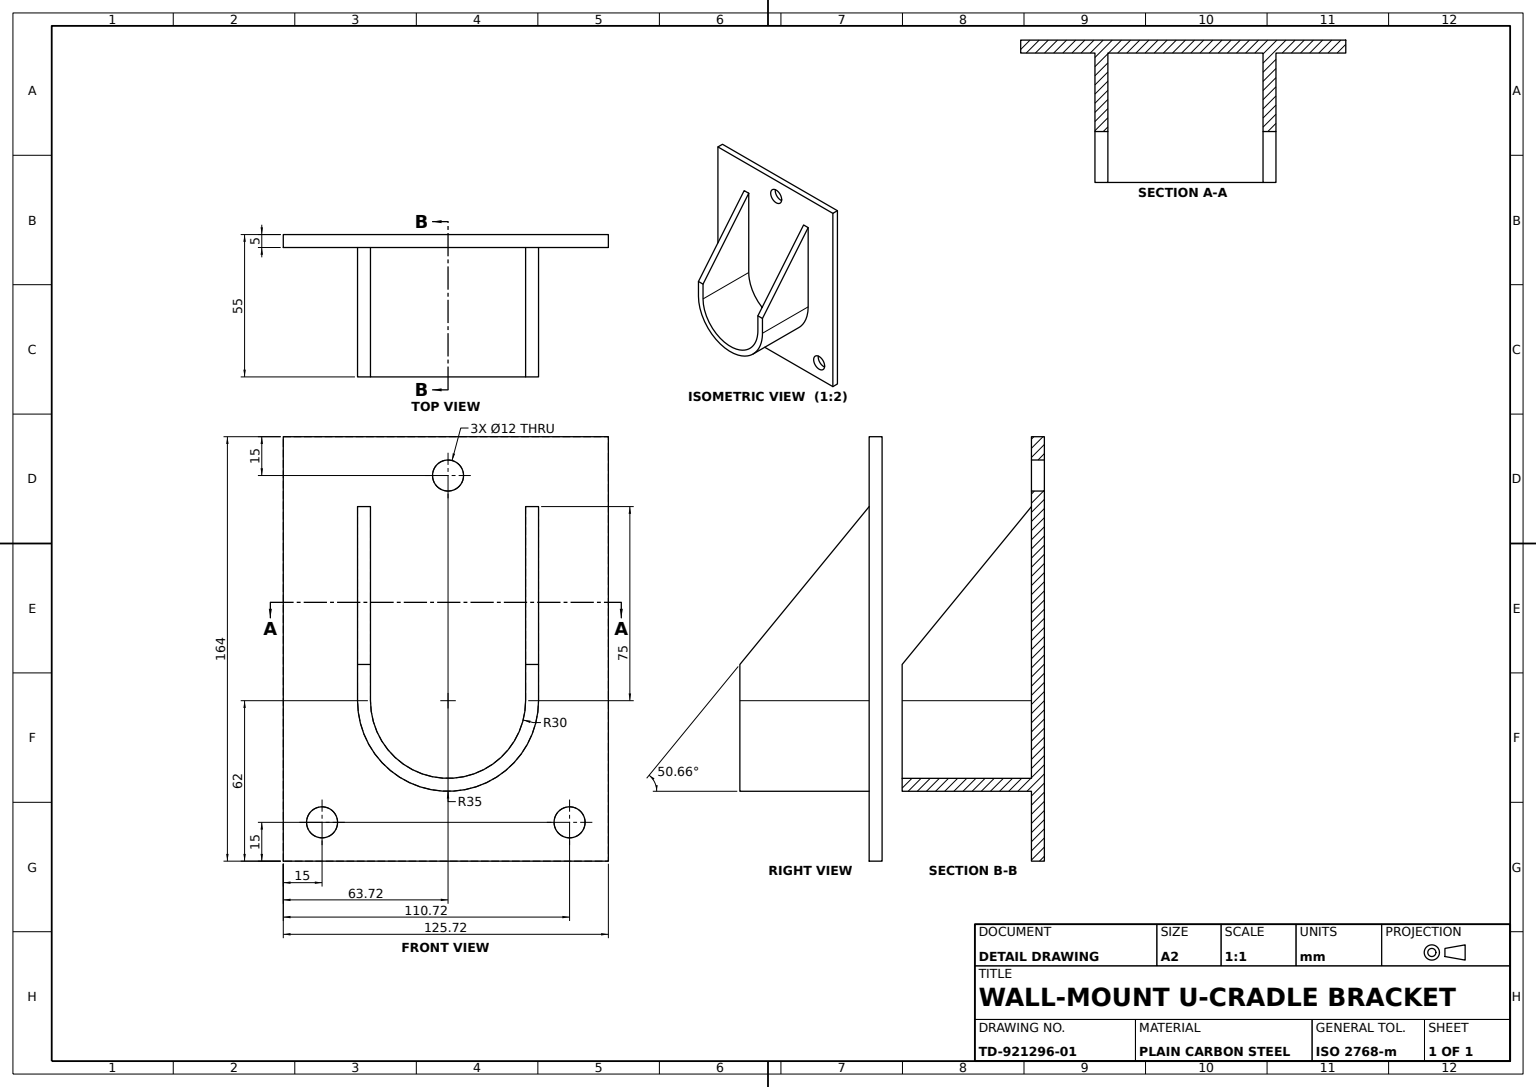
SolidWorks part; units mm, degrees
material "Plain Carbon Steel"
ref_plane "Front Plane" through (0, 0, 0) normal (0, 0, 1) x (1, 0, 0)
ref_plane "Top Plane" through (0, 0, 0) normal (0, 1, 0) x (1, 0, 0)
ref_plane "Right Plane" through (0, 0, 0) normal (1, 0, 0) x (0, 0, -1)
sketch "U-Channel Profile Sketch" plane through (0, 0, 0) normal (0, 0, 1) x (1, 0, 0)
  line L0 (0, 0) -> (0, 75) construction
  line L5 (35, 0) -> (35, 75)
  line L6 (-35, 0) -> (-35, 75)
  line L7 (30, 0) -> (30, 75)
  line L8 (-30, 0) -> (-30, 75)
  line L9 (-35, 75) -> (-30, 75)
  line L10 (30, 75) -> (35, 75)
  arc A4 (-35, 0) -> (35, 0) centre (0, 0) ccw
  arc A5 (-30, 0) -> (30, 0) centre (0, 0) ccw
  arc A6 (-25.7143, 15.4524) -> (25.7143, 15.4524) centre (0, 0) ccw construction
  arc A7 (-30, 18.0278) -> (30, 18.0278) centre (0, 0) ccw construction
  dimension "D3" = 35
  dimension "D6" = 5
  dimension "D1" = 75
extrude "U-Channel" add sketch "U-Channel Profile Sketch" along normal blind 55 contours L7 L10 L5 A4 L6 L9 L8 A5
sketch "Flange Plate Sketch" plane through (0, 0, 0) normal (0, 0, -1) x (-1, 0, 0)
  line L0 (-35, 0) -> (-35, 75) construction
  line L1 (-62, -62) -> (63.7173, -62)
  line L3 (-62, 102) -> (63.7173, 102)
  line L5 (-62, 102) -> (-62, -62)
  line L6 (63.7173, 102) -> (63.7173, -62)
  circle A1 centre (48.7173, -47) radius 6
  circle A2 centre (-47, -47) radius 6
  circle A3 centre (0, 87) radius 6
  point P0 (0, 0)
  dimension "D8" = 12
  dimension "D9" = 125.7173
  dimension "D1" = 62
  dimension "D2" = 102
  dimension "D3" = 15
  dimension "D4" = 15
  dimension "D5" = 15
  dimension "D6" = 15
  dimension "D7" = 15
  dimension "D10" = 83.7173
extrude "Flange Plate" add sketch "Flange Plate Sketch" against normal blind 5
sketch "Channel Side Trim Sketch" plane through (62, 0, 0) normal (1, 0, 0) x (0, 0, -1)
  line L1 (-55, 0) -> (-55, 75) construction
  line L2 (-55, 14) -> (-5, 75)
  line L3 (-5, 102) -> (-5, -62) construction
  line L4 (-5, 75) -> (-5, 0) construction
  line L7 (-5, 75) -> (-55, 75)
  line L8 (-55, 75) -> (-55, 14)
  line L10 (-5, 102) -> (0, 102) construction
  dimension "D1" = 27
  dimension "D2" = 88
extrude "Channel Side Trim" cut sketch "Channel Side Trim Sketch" against normal through all
